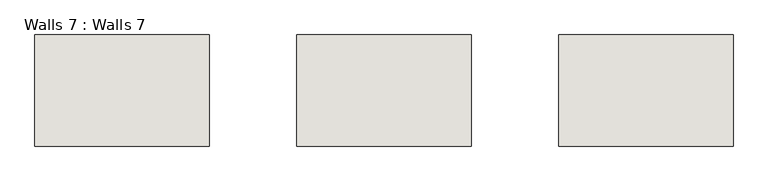
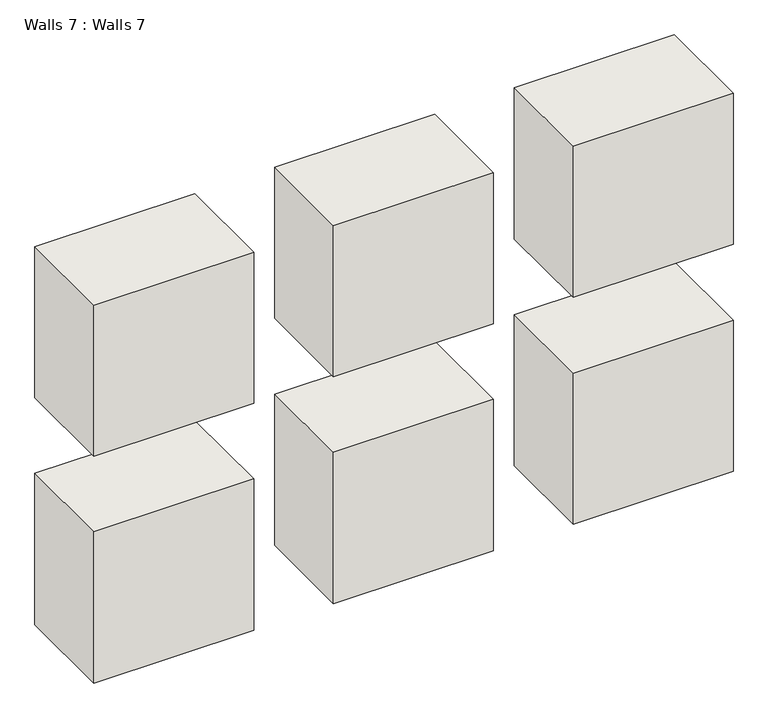
"""IFC4 building model written with IfcOpenShell, lengths in millimetres: wall geometry, Walls 7 : Walls 7."""

from ifc_helpers import new_model, si_unit, frame, origin, place, context, project, spatial, polyline, outline, extrude, source, transform, mapped, element, save


def walls_7_walls_7_e8c1ea63(model_context):
    return source(origin(), model_context, "Body", "SweptSolid", [
        extrude(outline(polyline([(-2913.0942714, 415.3135116), (-3217.8942714, 415.3135116), (-3217.8942714, 609.3081232), (-2913.0942714, 609.3081232), (-2913.0942714, 415.3135116)])), frame((0.0, 0.0, 854.1775432), z_axis=(0.0, 0.0, 1.0), x_axis=(1.0, 0.0, 0.0)), (0.0, 0.0, 1.0), 304.8),
        extrude(outline(polyline([(-2455.8942714, 415.3135116), (-2760.6942714, 415.3135116), (-2760.6942714, 609.3081232), (-2455.8942714, 609.3081232), (-2455.8942714, 415.3135116)])), frame((0.0, 0.0, 854.1775432), z_axis=(0.0, 0.0, 1.0), x_axis=(1.0, 0.0, 0.0)), (0.0, 0.0, 1.0), 304.8),
        extrude(outline(polyline([(-1998.6942714, 415.3135116), (-2303.4942714, 415.3135116), (-2303.4942714, 609.3081232), (-1998.6942714, 609.3081232), (-1998.6942714, 415.3135116)])), frame((0.0, 0.0, 854.1775432), z_axis=(0.0, 0.0, 1.0), x_axis=(1.0, 0.0, 0.0)), (0.0, 0.0, 1.0), 304.8),
        extrude(outline(polyline([(-2913.0942714, 415.3135116), (-3217.8942714, 415.3135116), (-3217.8942714, 609.3081232), (-2913.0942714, 609.3081232), (-2913.0942714, 415.3135116)])), frame((0.0, 0.0, 396.9775432), z_axis=(0.0, 0.0, 1.0), x_axis=(1.0, 0.0, 0.0)), (0.0, 0.0, 1.0), 304.8),
        extrude(outline(polyline([(-2455.8942714, 415.3135116), (-2760.6942714, 415.3135116), (-2760.6942714, 609.3081232), (-2455.8942714, 609.3081232), (-2455.8942714, 415.3135116)])), frame((0.0, 0.0, 396.9775432), z_axis=(0.0, 0.0, 1.0), x_axis=(1.0, 0.0, 0.0)), (0.0, 0.0, 1.0), 304.8),
        extrude(outline(polyline([(-1998.6942714, 415.3135116), (-2303.4942714, 415.3135116), (-2303.4942714, 609.3081232), (-1998.6942714, 609.3081232), (-1998.6942714, 415.3135116)])), frame((0.0, 0.0, 396.9775432), z_axis=(0.0, 0.0, 1.0), x_axis=(1.0, 0.0, 0.0)), (0.0, 0.0, 1.0), 304.8),
    ])


if __name__ == "__main__":
    model = new_model("IFC4")
    model_context = context("Model", 3, world=origin())
    ifc_project = project(units=[si_unit("LENGTHUNIT", "METRE", prefix="MILLI")], contexts=[model_context])
    site = spatial("IfcSite", under=ifc_project)
    building = spatial("IfcBuilding", under=site)
    placement = place(None, origin())
    walls_7_walls_7_shape = walls_7_walls_7_e8c1ea63(model_context)
    element("IfcWall", 1, ObjectType="Walls 7 : Walls 7", at=placement, inside=building, context=model_context, shape_type="MappedRepresentation", body=[
        mapped(walls_7_walls_7_shape, transform((0.0, 0.0, 0.0), x_axis=(1.0, 0.0, 0.0), y_axis=(0.0, 1.0, 0.0), z_axis=(0.0, 0.0, 1.0))),
    ])
    save(model, "model.ifc")

# Revit data of these elements
# Element 1 (IfcWall, "Walls 7 : Walls 7")
#   Materials on its faces: "Default Wall"
# Materials
#   "Default Wall": colour RGB 128 128 128, transparency 0
